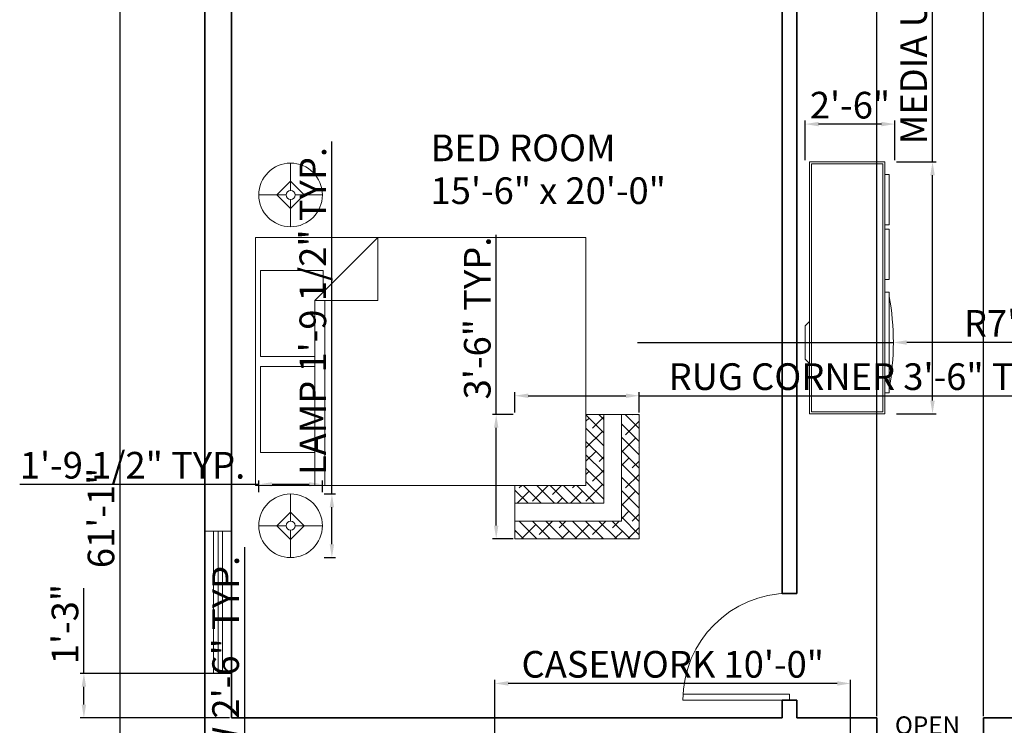
# Model space of a CAD drawing. Units: inches. Extents: x 1885 to 4781, y 1153 to 4395.
# Tile 3 of 7: x 2298 to 2631, y 1786 to 2024. Entities that reach past the tile are written whole.
import ezdxf

# ---------------------------------------------------------------- set-up
doc = ezdxf.new("R2010")
doc.units = ezdxf.units.IN
for name, color, linetype, lineweight in [('A-ANNO-DIMS', 5, 'Continuous', 18), ('A-FURN', 8, 'Continuous', 18), ('A-WALL', 7, 'Continuous', 35)]:
    doc.layers.add(name, color=color, linetype=linetype, lineweight=lineweight)
for name, color, linetype, lineweight, true_color in [('A-ANNO-TEXT', 244, 'Continuous', 18, 0x991b1e), ('A-AREA-IDEN', 244, 'Continuous', 18, 0x991b1e), ('A-DOOR', 11, 'Continuous', 18, 0xf27172), ('A-FLOR-PATT', 215, 'Continuous', 13, 0xa953a0), ('A-GLAZ', 152, 'Continuous', 18, 0x2776bb)]:
    doc.layers.add(name, color=color, linetype=linetype, lineweight=lineweight, true_color=true_color)
doc.styles.get("Standard").update_dxf_attribs({"font": 'arial.ttf'})
doc.dimstyles.new('ISO-25', dxfattribs={"dimtxt": 9, "dimasz": 4.5, "dimexe": 1.25, "dimexo": 0.625, "dimtad": 1, "dimdec": 0, "dimlunit": 3, "dimtxsty": 'Standard', "dimcen": 2.5, "dimadec": 0, "dimazin": 0, "dimtfac": 1, "dimtdec": 0, "dimtmove": 0, "dimatfit": 3, "dimfxl": 1, "dimarcsym": 0})

# ---------------------------------------------------------------- blocks, each defined once
blk = doc.blocks.new('Entertainment Center')
for p, q in [((-4, 0), (-5, -1)), ((4, 0), (-4, 0)), ((5, -1), (4, 0)), ((-17, -19), (-17, -1)), ((-17, -1), (43, -1)), ((-16.5, -18.5), (-16.5, -1.5)), ((-16.5, -1.5), (42.5, -1.5)), ((42.5, -1.5), (42.5, -18.5)), ((43, -1), (43, -19)), ((42.5, -18.5), (-16.5, -18.5)), ((43, -19), (-17, -19)), ((-12, -20), (-12, -19)), ((12, -20), (-12, -20)), ((12, -19), (12, -20)), ((15, -20), (15, -19)), ((27, -20), (15, -20)), ((27, -19), (27, -20)), ((28, -20), (28, -19)), ((40, -20), (28, -20)), ((40, -19), (40, -20))]:
    blk.add_line(p, q)
blk.add_arc((0, 40), 61, 259.6111, 280.3889)
blk = doc.blocks.new('Bed - Queen')
for p, q in [((0, -80.00003), (0, 0)), ((0, 0), (59.99999, 0)), ((59.99999, 0), (59.99999, -80.00003)), ((7.99999, -1.2), (28.79998, -1.2)), ((7.99999, -14.4), (7.99999, -1.2)), ((28.79998, -1.2), (28.79998, -14.4)), ((31.19999, -1.2), (51.99999, -1.2)), ((31.19999, -14.4), (31.19999, -1.2)), ((51.99999, -1.2), (51.99999, -16.4)), ((0, -14.4), (44.8, -14.4)), ((59.99999, -29.6), (44.8, -14.4)), ((44.8, -14.4), (44.8, -29.6)), ((51.99999, -16.4), (46.79936, -16.4)), ((44.8, -16.8), (0, -16.8)), ((44.8, -29.6), (59.99999, -29.6)), ((59.99999, -80.00003), (0, -80.00003))]:
    blk.add_line(p, q)
blk = doc.blocks.new('Lamp - Table')
for p, q in [((0, 7), (0, 1)), ((0, 3), (-3, 0)), ((3, 0), (0, 3)), ((-1, 0), (-7, 0)), ((-3, 0), (0, -3)), ((0, -3), (3, 0)), ((1, 0), (7, 0)), ((0, -1), (0, -7))]:
    blk.add_line(p, q)
for radius in [7, 1]:
    blk.add_circle((0, 0), radius)
blk = doc.blocks.new('*D26')
at = {"layer": 'A-ANNO-DIMS', "color": 0, "lineweight": -2, "transparency": 16777216}
for p, q in [((2360.28, 2222.42), (2331.02, 2222.42)), ((2332.27, 2217.92), (2332.27, 1493.92)), ((2360.28, 1489.42), (2331.02, 1489.42))]:
    blk.add_line(p, q, dxfattribs=at)
at = {"layer": 'A-ANNO-DIMS', "color": 0, "transparency": 16777216}
for points in [[(2331.52, 2217.92), (2333.02, 2217.92), (2332.27, 2222.42)], [(2331.52, 1493.92), (2333.02, 1493.92), (2332.27, 1489.42)]]:
    blk.add_solid(points, dxfattribs=at)
at = {"layer": 'Defpoints', "color": 0, "transparency": 16777216}
for p in [(2360.91, 2222.42), (2332.27, 1489.42), (2360.91, 1489.42)]:
    blk.add_point(p, dxfattribs=at)
at = {"layer": 'A-ANNO-DIMS', "color": 0, "transparency": 16777216, "insert": (2327.04, 1855.92), "char_height": 9, "attachment_point": 5, "rotation": 90}
blk.add_mtext('61\'-1"', dxfattribs=at)
blk = doc.blocks.new('WIN-48IN')
for p, q in [((0, 9), (48, 9)), ((0, 0), (0, 9)), ((48, 9), (48, 0)), ((0, 6), (48, 6)), ((0, 4.5), (48, 4.5)), ((0, 3), (48, 3)), ((48, 0), (0, 0))]:
    blk.add_line(p, q)
blk = doc.blocks.new('DOOR-SWING-36IN')
for p, q in [((0, 36), (0, 0)), ((2, 36), (2, 0)), ((0, 0), (2, 0))]:
    blk.add_line(p, q)
blk.add_arc((0, 0), 36, 0, 90)
blk = doc.blocks.new('RUG-CORNER-42IN')
for p, q in [((24, 18), (24, 42)), ((24, 42), (42, 42)), ((30, 42), (30, 12)), ((36, 42), (36, 6)), ((42, 42), (42, 0)), ((0, 0), (0, 18)), ((24, 18), (0, 18)), ((30, 12), (0, 12)), ((36, 6), (0, 6)), ((42, 0), (0, 0))]:
    blk.add_line(p, q)
blk = doc.blocks.new('*D33')
at = {"layer": 'A-ANNO-DIMS', "color": 0, "lineweight": -2, "transparency": 16777216}
for p, q in [((2403.87, 1864.01), (2403.87, 1982.93)), ((2401.28, 1864.01), (2405.12, 1864.01)), ((2403.87, 1847.02), (2403.87, 1859.51)), ((2401.28, 1842.52), (2405.12, 1842.52))]:
    blk.add_line(p, q, dxfattribs=at)
at = {"layer": 'A-ANNO-DIMS', "color": 0, "transparency": 16777216}
for points in [[(2403.12, 1859.51), (2404.62, 1859.51), (2403.87, 1864.01)], [(2403.12, 1847.02), (2404.62, 1847.02), (2403.87, 1842.52)]]:
    blk.add_solid(points, dxfattribs=at)
at = {"layer": 'Defpoints', "color": 0, "transparency": 16777216}
for p in [(2400.65, 1864.01), (2403.87, 1864.01), (2400.65, 1842.52)]:
    blk.add_point(p, dxfattribs=at)
at = {"layer": 'A-ANNO-DIMS', "color": 0, "transparency": 16777216, "insert": (2398.6, 1925.72), "char_height": 9, "attachment_point": 5, "rotation": 90}
blk.add_mtext('LAMP 1\'-9 1/2" TYP.', dxfattribs=at)
blk = doc.blocks.new('*D34')
at = {"layer": 'A-ANNO-DIMS', "color": 0, "lineweight": -2, "transparency": 16777216}
for p, q in [((2379.16, 1867.24), (2298.43, 1867.24)), ((2379.16, 1864.64), (2379.16, 1868.49)), ((2396.15, 1867.24), (2383.66, 1867.24)), ((2400.65, 1864.64), (2400.65, 1868.49))]:
    blk.add_line(p, q, dxfattribs=at)
at = {"layer": 'A-ANNO-DIMS', "color": 0, "transparency": 16777216}
for points in [[(2383.66, 1867.99), (2383.66, 1866.49), (2379.16, 1867.24)], [(2396.15, 1867.99), (2396.15, 1866.49), (2400.65, 1867.24)]]:
    blk.add_solid(points, dxfattribs=at)
at = {"layer": 'Defpoints', "color": 0, "transparency": 16777216}
for p in [(2379.16, 1867.24), (2379.16, 1864.01), (2400.65, 1864.01)]:
    blk.add_point(p, dxfattribs=at)
at = {"layer": 'A-ANNO-DIMS', "color": 0, "transparency": 16777216, "insert": (2336.54, 1872.52), "char_height": 9, "attachment_point": 5}
blk.add_mtext('1\'-9 1/2" TYP.', dxfattribs=at)
blk = doc.blocks.new('*D47')
at = {"layer": 'A-ANNO-DIMS', "color": 0, "lineweight": -2, "transparency": 16777216}
for p, q in [((2374.41, 1726.42), (2374.41, 1846.06)), ((2370.53, 1726.42), (2375.66, 1726.42)), ((2374.41, 1700.92), (2374.41, 1721.92)), ((2370.53, 1696.42), (2375.66, 1696.42))]:
    blk.add_line(p, q, dxfattribs=at)
at = {"layer": 'A-ANNO-DIMS', "color": 0, "transparency": 16777216}
for points in [[(2373.66, 1721.92), (2375.16, 1721.92), (2374.41, 1726.42)], [(2373.66, 1700.92), (2375.16, 1700.92), (2374.41, 1696.42)]]:
    blk.add_solid(points, dxfattribs=at)
at = {"layer": 'Defpoints', "color": 0, "transparency": 16777216}
for p in [(2369.91, 1726.42), (2374.41, 1726.42), (2369.91, 1696.42)]:
    blk.add_point(p, dxfattribs=at)
at = {"layer": 'A-ANNO-DIMS', "color": 0, "transparency": 16777216, "insert": (2369.13, 1788.49), "char_height": 9, "attachment_point": 5, "rotation": 90}
blk.add_mtext('WINDOW 2\'-6" TYP.', dxfattribs=at)
blk = doc.blocks.new('*D57')
at = {"layer": 'A-ANNO-DIMS', "color": 0, "lineweight": -2, "transparency": 16777216}
for p, q in [((2465.66, 1891.47), (2465.66, 1898.39)), ((2470.16, 1897.14), (2503.16, 1897.14)), ((2507.66, 1891.47), (2507.66, 1898.39)), ((2507.66, 1897.14), (2657.22, 1897.14))]:
    blk.add_line(p, q, dxfattribs=at)
at = {"layer": 'A-ANNO-DIMS', "color": 0, "transparency": 16777216}
for points in [[(2470.16, 1897.89), (2470.16, 1896.39), (2465.66, 1897.14)], [(2503.16, 1897.89), (2503.16, 1896.39), (2507.66, 1897.14)]]:
    blk.add_solid(points, dxfattribs=at)
at = {"layer": 'Defpoints', "color": 0, "transparency": 16777216}
for p in [(2507.66, 1897.14), (2465.66, 1890.84), (2507.66, 1890.84)]:
    blk.add_point(p, dxfattribs=at)
at = {"layer": 'A-ANNO-DIMS', "color": 0, "transparency": 16777216, "insert": (2584.69, 1902.43), "char_height": 9, "attachment_point": 5}
blk.add_mtext('RUG CORNER 3\'-6" TYP.', dxfattribs=at)
blk = doc.blocks.new('*D58')
at = {"layer": 'A-ANNO-DIMS', "color": 0, "lineweight": -2, "transparency": 16777216}
for p, q in [((2459.36, 1890.84), (2459.36, 1951.45)), ((2465.04, 1890.84), (2458.11, 1890.84)), ((2459.36, 1853.34), (2459.36, 1886.34)), ((2465.04, 1848.84), (2458.11, 1848.84))]:
    blk.add_line(p, q, dxfattribs=at)
at = {"layer": 'A-ANNO-DIMS', "color": 0, "transparency": 16777216}
for points in [[(2458.61, 1886.34), (2460.11, 1886.34), (2459.36, 1890.84)], [(2458.61, 1853.34), (2460.11, 1853.34), (2459.36, 1848.84)]]:
    blk.add_solid(points, dxfattribs=at)
at = {"layer": 'Defpoints', "color": 0, "transparency": 16777216}
for p in [(2459.36, 1890.84), (2465.66, 1890.84), (2465.66, 1848.84)]:
    blk.add_point(p, dxfattribs=at)
at = {"layer": 'A-ANNO-DIMS', "color": 0, "transparency": 16777216, "insert": (2454.14, 1923.39), "char_height": 9, "attachment_point": 5, "rotation": 90}
blk.add_mtext('3\'-6" TYP.', dxfattribs=at)
blk = doc.blocks.new('*D65')
at = {"layer": 'A-ANNO-DIMS', "color": 0, "lineweight": -2, "transparency": 16777216}
for p, q in [((2606.72, 1976.07), (2606.72, 2081.47)), ((2594.59, 1976.07), (2607.97, 1976.07)), ((2606.72, 1895.52), (2606.72, 1971.57)), ((2594.59, 1891.02), (2607.97, 1891.02))]:
    blk.add_line(p, q, dxfattribs=at)
at = {"layer": 'A-ANNO-DIMS', "color": 0, "transparency": 16777216}
for points in [[(2605.97, 1971.57), (2607.47, 1971.57), (2606.72, 1976.07)], [(2605.97, 1895.52), (2607.47, 1895.52), (2606.72, 1891.02)]]:
    blk.add_solid(points, dxfattribs=at)
at = {"layer": 'Defpoints', "color": 0, "transparency": 16777216}
for p in [(2593.97, 1976.07), (2606.72, 1976.07), (2593.97, 1891.02)]:
    blk.add_point(p, dxfattribs=at)
at = {"layer": 'A-ANNO-DIMS', "color": 0, "transparency": 16777216, "insert": (2601.5, 2031.02), "char_height": 9, "attachment_point": 5, "rotation": 90}
blk.add_mtext('MEDIA UNIT 7\'-1"', dxfattribs=at)
blk = doc.blocks.new('*D66')
at = {"layer": 'A-ANNO-DIMS', "color": 0, "lineweight": -2, "transparency": 16777216}
for p, q in [((2563.73, 1976.69), (2563.73, 1990.08)), ((2589.47, 1988.83), (2568.23, 1988.83)), ((2593.97, 1976.69), (2593.97, 1990.08))]:
    blk.add_line(p, q, dxfattribs=at)
at = {"layer": 'A-ANNO-DIMS', "color": 0, "transparency": 16777216}
for points in [[(2568.23, 1989.58), (2568.23, 1988.08), (2563.73, 1988.83)], [(2589.47, 1989.58), (2589.47, 1988.08), (2593.97, 1988.83)]]:
    blk.add_solid(points, dxfattribs=at)
at = {"layer": 'Defpoints', "color": 0, "transparency": 16777216}
for p in [(2563.73, 1988.83), (2563.73, 1976.07), (2593.97, 1976.07)]:
    blk.add_point(p, dxfattribs=at)
at = {"layer": 'A-ANNO-DIMS', "color": 0, "transparency": 16777216, "insert": (2578.85, 1994.05), "char_height": 9, "attachment_point": 5}
blk.add_mtext('2\'-6"', dxfattribs=at)
blk = doc.blocks.new('*D67')
at = {"layer": 'A-ANNO-DIMS', "color": 0, "lineweight": -2, "transparency": 16777216}
for p, q in [((2458.91, 1782.66), (2458.91, 1801.3)), ((2574.56, 1800.05), (2463.41, 1800.05)), ((2579.06, 1782.66), (2579.06, 1801.3))]:
    blk.add_line(p, q, dxfattribs=at)
at = {"layer": 'A-ANNO-DIMS', "color": 0, "transparency": 16777216}
for points in [[(2463.41, 1800.8), (2463.41, 1799.3), (2458.91, 1800.05)], [(2574.56, 1800.8), (2574.56, 1799.3), (2579.06, 1800.05)]]:
    blk.add_solid(points, dxfattribs=at)
at = {"layer": 'Defpoints', "color": 0, "transparency": 16777216}
for p in [(2458.91, 1800.05), (2458.91, 1782.03), (2579.06, 1782.03)]:
    blk.add_point(p, dxfattribs=at)
at = {"layer": 'A-ANNO-DIMS', "color": 0, "transparency": 16777216, "insert": (2518.99, 1805.34), "char_height": 9, "attachment_point": 5}
blk.add_mtext('CASEWORK 10\'-0"', dxfattribs=at)
blk = doc.blocks.new('*D85')
at = {"layer": 'A-ANNO-DIMS', "color": 0, "lineweight": -2, "transparency": 16777216}
for p, q in [((2320.11, 1803.42), (2320.11, 1832.24)), ((2369.28, 1803.42), (2318.86, 1803.42)), ((2320.11, 1792.92), (2320.11, 1798.92)), ((2369.28, 1788.42), (2318.86, 1788.42))]:
    blk.add_line(p, q, dxfattribs=at)
at = {"layer": 'A-ANNO-DIMS', "color": 0, "transparency": 16777216}
for points in [[(2319.36, 1798.92), (2320.86, 1798.92), (2320.11, 1803.42)], [(2319.36, 1792.92), (2320.86, 1792.92), (2320.11, 1788.42)]]:
    blk.add_solid(points, dxfattribs=at)
at = {"layer": 'Defpoints', "color": 0, "transparency": 16777216}
for p in [(2320.11, 1803.42), (2369.91, 1803.42), (2369.91, 1788.42)]:
    blk.add_point(p, dxfattribs=at)
at = {"layer": 'A-ANNO-DIMS', "color": 0, "transparency": 16777216, "insert": (2314.88, 1820.08), "char_height": 9, "attachment_point": 5, "rotation": 90}
blk.add_mtext('1\'-3"', dxfattribs=at)
blk = doc.blocks.new('*D90')
at = {"layer": 'A-ANNO-DIMS', "color": 0, "lineweight": -2, "transparency": 16777216}
for p, q in [((2587.91, 1789.05), (2587.91, 2264.47)), ((2592.41, 2263.22), (2619.41, 2263.22)), ((2623.91, 1789.05), (2623.91, 2264.47))]:
    blk.add_line(p, q, dxfattribs=at)
at = {"layer": 'A-ANNO-DIMS', "color": 0, "transparency": 16777216}
for points in [[(2592.41, 2263.97), (2592.41, 2262.47), (2587.91, 2263.22)], [(2619.41, 2263.97), (2619.41, 2262.47), (2623.91, 2263.22)]]:
    blk.add_solid(points, dxfattribs=at)
at = {"layer": 'Defpoints', "color": 0, "transparency": 16777216}
for p in [(2623.91, 2263.22), (2587.91, 1788.42), (2623.91, 1788.42)]:
    blk.add_point(p, dxfattribs=at)
at = {"layer": 'A-ANNO-DIMS', "color": 0, "transparency": 16777216, "insert": (2605.91, 2268.44), "char_height": 9, "attachment_point": 5}
blk.add_mtext('3\'-0"', dxfattribs=at)
blk = doc.blocks.new('*D97')
at = {"layer": 'A-ANNO-DIMS', "color": 0, "lineweight": -2, "transparency": 16777216}
for p, q in [((2507.03, 1915.12), (2593.49, 1915.12)), ((2672.75, 1915.12), (2597.99, 1915.12))]:
    blk.add_line(p, q, dxfattribs=at)
at = {"layer": 'A-ANNO-DIMS', "color": 0, "transparency": 16777216}
blk.add_solid([(2597.99, 1915.87), (2597.99, 1914.37), (2593.49, 1915.12)], dxfattribs=at)
at = {"layer": 'Defpoints', "color": 0, "transparency": 16777216}
for p in [(2507.03, 1915.12), (2593.49, 1915.12)]:
    blk.add_point(p, dxfattribs=at)
at = {"layer": 'A-ANNO-DIMS', "color": 0, "transparency": 16777216, "insert": (2645.37, 1920.4), "char_height": 9, "attachment_point": 5, "rotation": 0.0003}
blk.add_mtext('R7\'-2 1/2"', dxfattribs=at)

msp = doc.modelspace()

# ---------------------------------------------------------------- hatches: boundary and pattern name
at = {"layer": 'A-FLOR-PATT'}
h = msp.add_hatch(dxfattribs=at)
h.set_pattern_fill('ANSI38', color=256, angle=90)
h.set_pattern_definition([(135, (4583.1316, -741.618), (-2.245064, -2.245064), []), (225, (4583.1316, -741.618), (-2.245064, -6.735192), [7.9375, -4.7625])])
h.paths.add_polyline_path([(2465.66, 1860.84), (2465.66, 1866.84), (2489.66, 1866.84), (2489.66, 1890.84), (2495.66, 1890.84), (2495.66, 1860.84)], flags=17)
h.paths.add_polyline_path([(2465.66, 1848.84), (2465.66, 1854.84), (2501.66, 1854.84), (2501.66, 1890.84), (2507.66, 1890.84), (2507.66, 1848.84)])

# ---------------------------------------------------------------- linework, layer by layer
at = {"layer": 'A-WALL'}
for p, q in [((2360.91, 2222.42), (2360.91, 1489.42)), ((2369.91, 2028.42), (2369.91, 1788.42)), ((2555.91, 2028.42), (2555.91, 1830.42)), ((2560.91, 2028.42), (2560.91, 1830.42)), ((2555.91, 1830.42), (2560.91, 1830.42)), ((2555.91, 1794.42), (2555.91, 1788.42)), ((2555.91, 1794.42), (2560.91, 1794.42)), ((2560.91, 1794.42), (2560.91, 1788.42)), ((2369.91, 1788.42), (2555.91, 1788.42)), ((2560.91, 1788.42), (2587.91, 1788.42)), ((2587.91, 1788.42), (2587.91, 1783.42)), ((2623.91, 1788.42), (2623.91, 1783.42)), ((2623.91, 1788.42), (2643.91, 1788.42))]:
    msp.add_line(p, q, dxfattribs=at)

# ---------------------------------------------------------------- block references
at = {"layer": 'A-DOOR', "rotation": 89.9999999999992}
msp.add_blockref('DOOR-SWING-36IN', (2558.41, 1794.42), dxfattribs=at)
at = {"layer": 'A-FURN', "rotation": 90}
for name, p, xscale, yscale, zscale in [('Lamp - Table', (2389.91, 1964.92), 1.53498639786184, 1.53498639786184, 1.53498639786184), ('Entertainment Center', (2563.73, 1915.12), 1.417473391607583, 1.417473391607583, 1.417473391607583), ('Bed - Queen', (2378.06, 1866.84), 1.395073646196092, 1.395073646196092, 1.395073646196092), ('Lamp - Table', (2389.91, 1853.27), 1.53498639786184, 1.53498639786184, 1.53498639786184)]:
    msp.add_blockref(name, p, dxfattribs=dict(at, xscale=xscale, yscale=yscale, zscale=zscale))
at = {"layer": 'A-FURN'}
msp.add_blockref('RUG-CORNER-42IN', (2465.66, 1848.84), dxfattribs=at)
at = {"layer": 'A-GLAZ', "rotation": 90.00000000000179}
msp.add_blockref('WIN-48IN', (2369.91, 1803.42), dxfattribs=at)

# ---------------------------------------------------------------- texts
at = {"layer": 'A-ANNO-TEXT'}
msp.add_text('OPEN', height=6, dxfattribs=at).set_placement((2594.03, 1782.93))
at = {"layer": 'A-AREA-IDEN'}
for s, p in [('BED ROOM', (2437.19, 1976.31)), ('15\'-6" x 20\'-0"', (2437.19, 1961.85))]:
    msp.add_text(s, height=9, dxfattribs=at).set_placement(p)

# ---------------------------------------------------------------- dimensions: what is measured, and where the dimension line sits
at = {"layer": 'A-ANNO-DIMS'}
dim = msp.add_linear_dim(base=(2623.91, 2263.22), p1=(2587.91, 1788.42), p2=(2623.91, 1788.42), dimstyle='ISO-25', override={"dimdec": 1, "dimlfac": 1, "dimrnd": 0, "dimzin": 1, "dimdsep": 46, "dimlunit": 4, "dimfrac": 2}, dxfattribs=at)
dim.commit()
dim.dimension.update_dxf_attribs({"geometry": '*D90', "text_midpoint": (2605.91, 2268.44)})
for base, p1, p2, angle, override, picture, middle in [((2332.27, 1489.42), (2360.91, 2222.42), (2360.91, 1489.42), 90, {"dimclrd": 0, "dimclre": 0, "dimclrt": 0}, '*D26', (2327.04, 1855.92)), ((2563.73, 1988.83), (2593.97, 1976.07), (2563.73, 1976.07), 180, {"dimdec": 1, "dimlfac": 1, "dimrnd": 0, "dimzin": 1, "dimdsep": 46, "dimlunit": 4, "dimfrac": 2}, '*D66', (2578.85, 1994.05)), ((2320.11, 1803.42), (2369.91, 1788.42), (2369.91, 1803.42), 90, {"dimdec": 1, "dimlfac": 1, "dimrnd": 0, "dimzin": 1, "dimdsep": 46, "dimlunit": 4, "dimfrac": 2}, '*D85', (2314.88, 1820.08))]:
    dim = msp.add_linear_dim(base=base, p1=p1, p2=p2, angle=angle, dimstyle='ISO-25', override=override, dxfattribs=at)
    dim.commit()
    dim.dimension.update_dxf_attribs({"geometry": picture, "text_midpoint": middle})
for base, p1, p2, angle, text, picture, middle in [((2606.7226, 1976.0689), (2593.9653, 1891.0205), (2593.9653, 1976.0689), 90, 'MEDIA UNIT <>', '*D65', (2601.5024, 2031.0193)), ((2403.87, 1864.01), (2400.65, 1842.52), (2400.65, 1864.01), 90, 'LAMP <> TYP.', '*D33', (2398.6, 1925.72)), ((2459.36, 1890.84), (2465.66, 1848.84), (2465.66, 1890.84), 90, '<> TYP.', '*D58', (2454.14, 1923.39)), ((2379.16, 1867.24), (2400.65, 1864.01), (2379.16, 1864.01), 180, '<> TYP.', '*D34', (2336.54, 1872.52)), ((2374.41, 1726.42), (2369.91, 1696.42), (2369.91, 1726.42), 90, 'WINDOW <> TYP.', '*D47', (2369.13, 1788.49)), ((2458.9075, 1800.0546), (2579.0628, 1782.0313), (2458.9075, 1782.0313), 180, 'CASEWORK <>', '*D67', (2518.9851, 1805.3361))]:
    dim = msp.add_linear_dim(base=base, p1=p1, p2=p2, angle=angle, text=text, dimstyle='ISO-25', override={"dimdec": 1, "dimlfac": 1, "dimrnd": 0, "dimzin": 1, "dimdsep": 46, "dimlunit": 4, "dimfrac": 2}, dxfattribs=at)
    dim.commit()
    dim.dimension.update_dxf_attribs({"geometry": picture, "text_midpoint": middle})
dim = msp.add_radius_dim(center=(2507.03, 1915.12), mpoint=(2593.49, 1915.12), dimstyle='ISO-25', override={"dimdec": 1, "dimlfac": 1, "dimrnd": 0, "dimzin": 1, "dimdsep": 46, "dimlunit": 4, "dimfrac": 2}, dxfattribs=at)
dim.commit()
dim.dimension.update_dxf_attribs({"geometry": '*D97', "text_midpoint": (2645.37, 1915.12), "dimtype": 164})
dim = msp.add_linear_dim(base=(2507.66, 1897.14), p1=(2465.66, 1890.84), p2=(2507.66, 1890.84), text='RUG CORNER <> TYP.', dimstyle='ISO-25', override={"dimdec": 1, "dimlfac": 1, "dimrnd": 0, "dimzin": 1, "dimdsep": 46, "dimlunit": 4, "dimfrac": 2}, dxfattribs=at)
dim.commit()
dim.dimension.update_dxf_attribs({"geometry": '*D57', "text_midpoint": (2584.69, 1902.43)})

doc.saveas('drawing.dxf')
